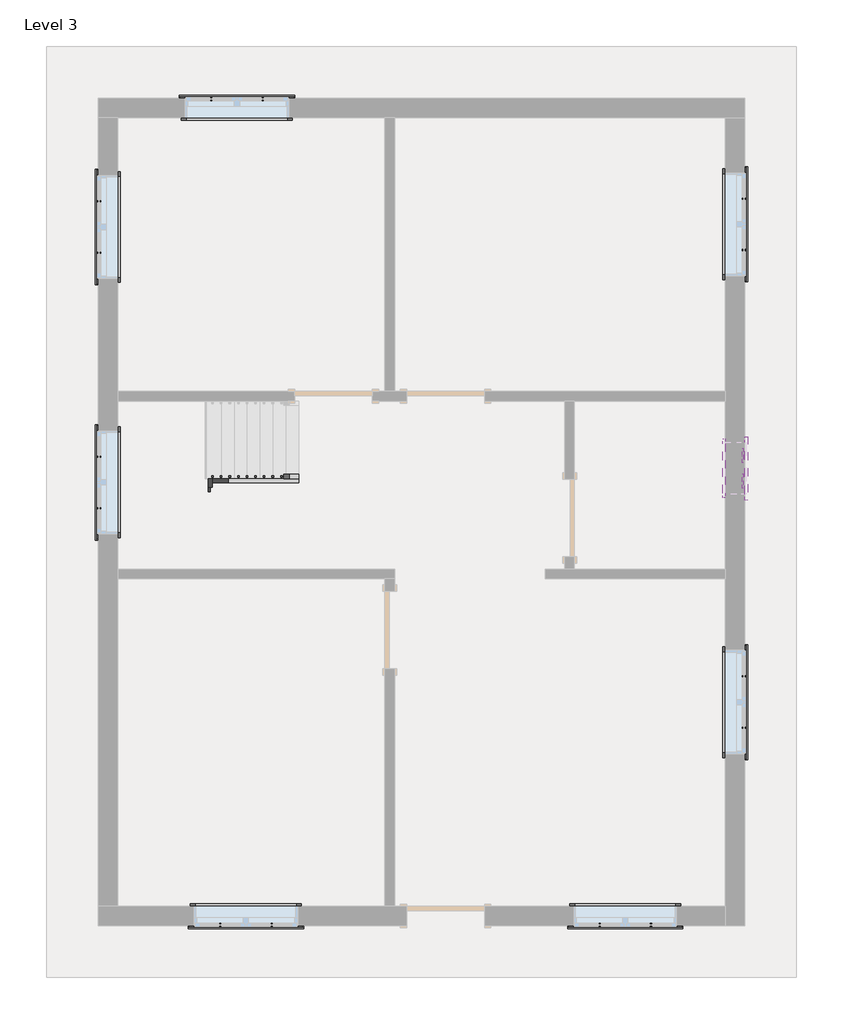
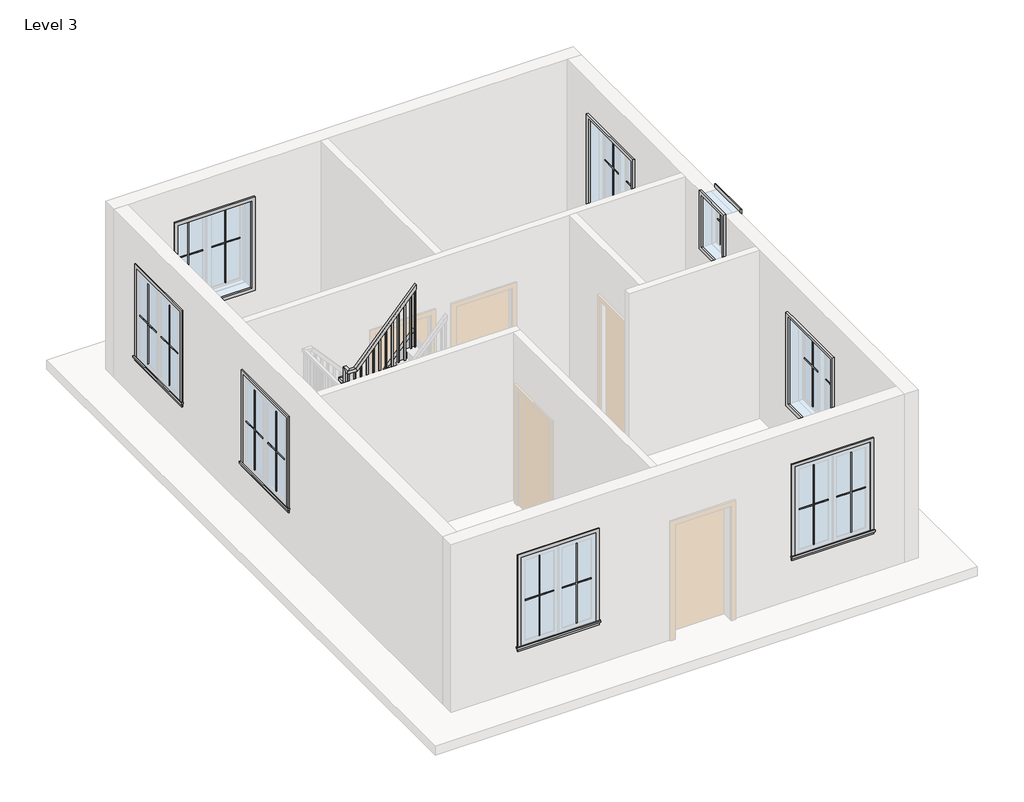
# One storey, part 2 of 2: 32 proxies, 3 members, 1 railing.
"""IFC4 building model written with IfcOpenShell, lengths in millimetres."""

from ifc_helpers import new_model, si_unit, frame, origin, place, context, project, spatial, polyline, outline, extrude, faceted_brep, transform, mapped, element, save
from components import muntin_pattern_2x2_muntin_pattern_2x2_6dad3731, muntin_pattern_2x2_muntin_pattern_2x2_a30a3345, muntin_pattern_2x2_muntin_pattern_2x2_53152e2c, muntin_pattern_2x2_muntin_pattern_2x2_e8f3e573, trim_window_exterior_flat_with_sill_92b9b949, trim_window_exterior_flat_with_sill_a665a915, trim_window_interior_flat_picture_frame_3bb882cf, trim_window_interior_flat_picture_frame_d485c387

model = new_model("IFC4")

# Units and contexts
model_context = context("Model", 3, world=origin())
ifc_project = project(units=[si_unit("LENGTHUNIT", "METRE", prefix="MILLI")], contexts=[model_context])

# Site, building, storey
site = spatial("IfcSite", under=ifc_project)
building = spatial("IfcBuilding", under=site)
storey = spatial("IfcBuildingStorey", under=building, Name="Level 3", Elevation=6096.0)

# Proxies
placement = place(None, origin())
muntin_pattern_2x2_muntin_pattern_2x2_shape = muntin_pattern_2x2_muntin_pattern_2x2_6dad3731(model_context)
element("IfcBuildingElementProxy", 1, Name="Muntin Pattern_2x2 : Muntin Pattern_2x2", ObjectType="Muntin Pattern_2x2 : Muntin Pattern_2x2", at=placement, inside=storey, context=model_context, shape_type="MappedRepresentation", body=[
    mapped(muntin_pattern_2x2_muntin_pattern_2x2_shape, transform((7785.1, 4733.925, 7080.25), x_axis=(-1.0, 0.0, 0.0), y_axis=(0.0, -1.0, 0.0), z_axis=(0.0, 0.0, 1.0))),
])
element("IfcBuildingElementProxy", 2, Name="Muntin Pattern_2x2 : Muntin Pattern_2x2", ObjectType="Muntin Pattern_2x2 : Muntin Pattern_2x2", at=placement, inside=storey, context=model_context, shape_type="MappedRepresentation", body=[
    mapped(muntin_pattern_2x2_muntin_pattern_2x2_shape, transform((3313.1125, 4733.925, 7080.25), x_axis=(-1.0, 0.0, 0.0), y_axis=(0.0, -1.0, 0.0), z_axis=(0.0, 0.0, 1.0))),
])
element("IfcBuildingElementProxy", 3, Name="Muntin Pattern_2x2 : Muntin Pattern_2x2", ObjectType="Muntin Pattern_2x2 : Muntin Pattern_2x2", at=placement, inside=storey, context=model_context, shape_type="MappedRepresentation", body=[
    mapped(muntin_pattern_2x2_muntin_pattern_2x2_shape, transform((8880.475, 13295.3125, 7080.25), x_axis=(0.0, -1.0, 0.0), y_axis=(1.0, 0.0, 0.0), z_axis=(0.0, 0.0, 1.0))),
])
element("IfcBuildingElementProxy", 4, Name="Muntin Pattern_2x2 : Muntin Pattern_2x2", ObjectType="Muntin Pattern_2x2 : Muntin Pattern_2x2", at=placement, inside=storey, context=model_context, shape_type="MappedRepresentation", body=[
    mapped(muntin_pattern_2x2_muntin_pattern_2x2_shape, transform((8880.475, 7662.8625, 7080.25), x_axis=(0.0, -1.0, 0.0), y_axis=(1.0, 0.0, 0.0), z_axis=(0.0, 0.0, 1.0))),
])
element("IfcBuildingElementProxy", 5, Name="Muntin Pattern_2x2 : Muntin Pattern_2x2", ObjectType="Muntin Pattern_2x2 : Muntin Pattern_2x2", at=placement, inside=storey, context=model_context, shape_type="MappedRepresentation", body=[
    mapped(muntin_pattern_2x2_muntin_pattern_2x2_shape, transform((1279.525, 12657.1375, 7080.25), x_axis=(0.0, 1.0, 0.0), y_axis=(-1.0, 0.0, 0.0), z_axis=(0.0, 0.0, 1.0))),
])
element("IfcBuildingElementProxy", 6, Name="Muntin Pattern_2x2 : Muntin Pattern_2x2", ObjectType="Muntin Pattern_2x2 : Muntin Pattern_2x2", at=placement, inside=storey, context=model_context, shape_type="MappedRepresentation", body=[
    mapped(muntin_pattern_2x2_muntin_pattern_2x2_shape, transform((1279.525, 9647.2375, 7080.25), x_axis=(0.0, 1.0, 0.0), y_axis=(-1.0, 0.0, 0.0), z_axis=(0.0, 0.0, 1.0))),
])
element("IfcBuildingElementProxy", 7, Name="Muntin Pattern_2x2 : Muntin Pattern_2x2", ObjectType="Muntin Pattern_2x2 : Muntin Pattern_2x2", at=placement, inside=storey, context=model_context, shape_type="MappedRepresentation", body=[
    mapped(muntin_pattern_2x2_muntin_pattern_2x2_shape, transform((2601.9125, 14468.475, 7080.25), x_axis=(1.0, 0.0, 0.0), y_axis=(0.0, 1.0, 0.0), z_axis=(0.0, 0.0, 1.0))),
])
muntin_pattern_2x2_muntin_pattern_2x2_2_shape = muntin_pattern_2x2_muntin_pattern_2x2_a30a3345(model_context)
element("IfcBuildingElementProxy", 8, Name="Muntin Pattern_2x2 : Muntin Pattern_2x2", ObjectType="Muntin Pattern_2x2 : Muntin Pattern_2x2", at=placement, inside=storey, context=model_context, shape_type="MappedRepresentation", body=[
    mapped(muntin_pattern_2x2_muntin_pattern_2x2_2_shape, transform((7178.675, 4733.925, 7080.25), x_axis=(1.0, 0.0, 0.0), y_axis=(0.0, 1.0, 0.0), z_axis=(0.0, 0.0, 1.0))),
])
element("IfcBuildingElementProxy", 9, Name="Muntin Pattern_2x2 : Muntin Pattern_2x2", ObjectType="Muntin Pattern_2x2 : Muntin Pattern_2x2", at=placement, inside=storey, context=model_context, shape_type="MappedRepresentation", body=[
    mapped(muntin_pattern_2x2_muntin_pattern_2x2_2_shape, transform((2706.6875, 4733.925, 7080.25), x_axis=(1.0, 0.0, 0.0), y_axis=(0.0, 1.0, 0.0), z_axis=(0.0, 0.0, 1.0))),
])
element("IfcBuildingElementProxy", 10, Name="Muntin Pattern_2x2 : Muntin Pattern_2x2", ObjectType="Muntin Pattern_2x2 : Muntin Pattern_2x2", at=placement, inside=storey, context=model_context, shape_type="MappedRepresentation", body=[
    mapped(muntin_pattern_2x2_muntin_pattern_2x2_2_shape, transform((8880.475, 12688.8875, 7080.25), x_axis=(0.0, 1.0, 0.0), y_axis=(-1.0, 0.0, 0.0), z_axis=(0.0, 0.0, 1.0))),
])
element("IfcBuildingElementProxy", 11, Name="Muntin Pattern_2x2 : Muntin Pattern_2x2", ObjectType="Muntin Pattern_2x2 : Muntin Pattern_2x2", at=placement, inside=storey, context=model_context, shape_type="MappedRepresentation", body=[
    mapped(muntin_pattern_2x2_muntin_pattern_2x2_2_shape, transform((8880.475, 7056.4375, 7080.25), x_axis=(0.0, 1.0, 0.0), y_axis=(-1.0, 0.0, 0.0), z_axis=(0.0, 0.0, 1.0))),
])
element("IfcBuildingElementProxy", 12, Name="Muntin Pattern_2x2 : Muntin Pattern_2x2", ObjectType="Muntin Pattern_2x2 : Muntin Pattern_2x2", at=placement, inside=storey, context=model_context, shape_type="MappedRepresentation", body=[
    mapped(muntin_pattern_2x2_muntin_pattern_2x2_2_shape, transform((1279.525, 13263.5625, 7080.25), x_axis=(0.0, -1.0, 0.0), y_axis=(1.0, 0.0, 0.0), z_axis=(0.0, 0.0, 1.0))),
])
element("IfcBuildingElementProxy", 13, Name="Muntin Pattern_2x2 : Muntin Pattern_2x2", ObjectType="Muntin Pattern_2x2 : Muntin Pattern_2x2", at=placement, inside=storey, context=model_context, shape_type="MappedRepresentation", body=[
    mapped(muntin_pattern_2x2_muntin_pattern_2x2_2_shape, transform((1279.525, 10253.6625, 7080.25), x_axis=(0.0, -1.0, 0.0), y_axis=(1.0, 0.0, 0.0), z_axis=(0.0, 0.0, 1.0))),
])
element("IfcBuildingElementProxy", 14, Name="Muntin Pattern_2x2 : Muntin Pattern_2x2", ObjectType="Muntin Pattern_2x2 : Muntin Pattern_2x2", at=placement, inside=storey, context=model_context, shape_type="MappedRepresentation", body=[
    mapped(muntin_pattern_2x2_muntin_pattern_2x2_2_shape, transform((3208.3375, 14468.475, 7080.25), x_axis=(-1.0, 0.0, 0.0), y_axis=(0.0, -1.0, 0.0), z_axis=(0.0, 0.0, 1.0))),
])
muntin_pattern_2x2_muntin_pattern_2x2_3_shape = muntin_pattern_2x2_muntin_pattern_2x2_53152e2c(model_context)
element("IfcBuildingElementProxy", 15, Name="Muntin Pattern_2x2 : Muntin Pattern_2x2", ObjectType="Muntin Pattern_2x2 : Muntin Pattern_2x2", at=placement, inside=storey, context=model_context, shape_type="MappedRepresentation", body=[
    mapped(muntin_pattern_2x2_muntin_pattern_2x2_3_shape, transform((8880.475, 10266.3625, 8299.45), x_axis=(0.0, -1.0, 0.0), y_axis=(1.0, 0.0, 0.0), z_axis=(0.0, 0.0, 1.0))),
])
muntin_pattern_2x2_muntin_pattern_2x2_4_shape = muntin_pattern_2x2_muntin_pattern_2x2_e8f3e573(model_context)
element("IfcBuildingElementProxy", 16, Name="Muntin Pattern_2x2 : Muntin Pattern_2x2", ObjectType="Muntin Pattern_2x2 : Muntin Pattern_2x2", at=placement, inside=storey, context=model_context, shape_type="MappedRepresentation", body=[
    mapped(muntin_pattern_2x2_muntin_pattern_2x2_4_shape, transform((8880.475, 9964.7375, 8299.45), x_axis=(0.0, 1.0, 0.0), y_axis=(-1.0, 0.0, 0.0), z_axis=(0.0, 0.0, 1.0))),
])
trim_window_exterior_flat_with_sill_shape = trim_window_exterior_flat_with_sill_92b9b949(model_context)
element("IfcBuildingElementProxy", 17, Name="Trim-Window-Exterior-Flat : with Sill", ObjectType="Trim-Window-Exterior-Flat : with Sill", at=placement, inside=storey, context=model_context, shape_type="MappedRepresentation", body=[
    mapped(trim_window_exterior_flat_with_sill_shape, transform((7481.8875, 4724.4, 8534.4), x_axis=(1.0, 0.0, 0.0), y_axis=(0.0, 0.0, 1.0), z_axis=(0.0, -1.0, 0.0))),
])
element("IfcBuildingElementProxy", 18, Name="Trim-Window-Exterior-Flat : with Sill", ObjectType="Trim-Window-Exterior-Flat : with Sill", at=placement, inside=storey, context=model_context, shape_type="MappedRepresentation", body=[
    mapped(trim_window_exterior_flat_with_sill_shape, transform((3009.9, 4724.4, 8534.4), x_axis=(1.0, 0.0, 0.0), y_axis=(0.0, 0.0, 1.0), z_axis=(0.0, -1.0, 0.0))),
])
element("IfcBuildingElementProxy", 19, Name="Trim-Window-Exterior-Flat : with Sill", ObjectType="Trim-Window-Exterior-Flat : with Sill", at=placement, inside=storey, context=model_context, shape_type="MappedRepresentation", body=[
    mapped(trim_window_exterior_flat_with_sill_shape, transform((8890.0, 12992.1, 8534.4), x_axis=(0.0, 1.0, 0.0), y_axis=(0.0, 0.0, 1.0), z_axis=(1.0, 0.0, 0.0))),
])
element("IfcBuildingElementProxy", 20, Name="Trim-Window-Exterior-Flat : with Sill", ObjectType="Trim-Window-Exterior-Flat : with Sill", at=placement, inside=storey, context=model_context, shape_type="MappedRepresentation", body=[
    mapped(trim_window_exterior_flat_with_sill_shape, transform((8890.0, 7359.65, 8534.4), x_axis=(0.0, 1.0, 0.0), y_axis=(0.0, 0.0, 1.0), z_axis=(1.0, 0.0, 0.0))),
])
element("IfcBuildingElementProxy", 21, Name="Trim-Window-Exterior-Flat : with Sill", ObjectType="Trim-Window-Exterior-Flat : with Sill", at=placement, inside=storey, context=model_context, shape_type="MappedRepresentation", body=[
    mapped(trim_window_exterior_flat_with_sill_shape, transform((1270.0, 12960.35, 8534.4), x_axis=(0.0, -1.0, 0.0), y_axis=(0.0, 0.0, 1.0), z_axis=(-1.0, 0.0, 0.0))),
])
element("IfcBuildingElementProxy", 22, Name="Trim-Window-Exterior-Flat : with Sill", ObjectType="Trim-Window-Exterior-Flat : with Sill", at=placement, inside=storey, context=model_context, shape_type="MappedRepresentation", body=[
    mapped(trim_window_exterior_flat_with_sill_shape, transform((1270.0, 9950.45, 8534.4), x_axis=(0.0, -1.0, 0.0), y_axis=(0.0, 0.0, 1.0), z_axis=(-1.0, 0.0, 0.0))),
])
element("IfcBuildingElementProxy", 23, Name="Trim-Window-Exterior-Flat : with Sill", ObjectType="Trim-Window-Exterior-Flat : with Sill", at=placement, inside=storey, context=model_context, shape_type="MappedRepresentation", body=[
    mapped(trim_window_exterior_flat_with_sill_shape, transform((2905.125, 14478.0, 8534.4), x_axis=(-1.0, 0.0, 0.0), y_axis=(0.0, 0.0, 1.0), z_axis=(0.0, 1.0, 0.0))),
])
trim_window_exterior_flat_with_sill_2_shape = trim_window_exterior_flat_with_sill_a665a915(model_context)
element("IfcBuildingElementProxy", 24, Name="Trim-Window-Exterior-Flat : with Sill", ObjectType="Trim-Window-Exterior-Flat : with Sill", at=placement, inside=storey, context=model_context, shape_type="MappedRepresentation", body=[
    mapped(trim_window_exterior_flat_with_sill_2_shape, transform((8890.0, 10115.55, 9144.0), x_axis=(0.0, 1.0, 0.0), y_axis=(0.0, 0.0, 1.0), z_axis=(1.0, 0.0, 0.0))),
])
trim_window_interior_flat_picture_frame_shape = trim_window_interior_flat_picture_frame_3bb882cf(model_context)
element("IfcBuildingElementProxy", 25, Name="Trim-Window-Interior-Flat : Picture Frame", ObjectType="Trim-Window-Interior-Flat : Picture Frame", at=placement, inside=storey, context=model_context, shape_type="MappedRepresentation", body=[
    mapped(trim_window_interior_flat_picture_frame_shape, transform((7481.8875, 4953.0, 8534.4), x_axis=(-1.0, 0.0, 0.0), y_axis=(0.0, 0.0, 1.0), z_axis=(0.0, 1.0, 0.0))),
])
element("IfcBuildingElementProxy", 26, Name="Trim-Window-Interior-Flat : Picture Frame", ObjectType="Trim-Window-Interior-Flat : Picture Frame", at=placement, inside=storey, context=model_context, shape_type="MappedRepresentation", body=[
    mapped(trim_window_interior_flat_picture_frame_shape, transform((3009.9, 4953.0, 8534.4), x_axis=(-1.0, 0.0, 0.0), y_axis=(0.0, 0.0, 1.0), z_axis=(0.0, 1.0, 0.0))),
])
element("IfcBuildingElementProxy", 27, Name="Trim-Window-Interior-Flat : Picture Frame", ObjectType="Trim-Window-Interior-Flat : Picture Frame", at=placement, inside=storey, context=model_context, shape_type="MappedRepresentation", body=[
    mapped(trim_window_interior_flat_picture_frame_shape, transform((8661.4, 12992.1, 8534.4), x_axis=(0.0, -1.0, 0.0), y_axis=(0.0, 0.0, 1.0), z_axis=(-1.0, 0.0, 0.0))),
])
element("IfcBuildingElementProxy", 28, Name="Trim-Window-Interior-Flat : Picture Frame", ObjectType="Trim-Window-Interior-Flat : Picture Frame", at=placement, inside=storey, context=model_context, shape_type="MappedRepresentation", body=[
    mapped(trim_window_interior_flat_picture_frame_shape, transform((8661.4, 7359.65, 8534.4), x_axis=(0.0, -1.0, 0.0), y_axis=(0.0, 0.0, 1.0), z_axis=(-1.0, 0.0, 0.0))),
])
element("IfcBuildingElementProxy", 29, Name="Trim-Window-Interior-Flat : Picture Frame", ObjectType="Trim-Window-Interior-Flat : Picture Frame", at=placement, inside=storey, context=model_context, shape_type="MappedRepresentation", body=[
    mapped(trim_window_interior_flat_picture_frame_shape, transform((1498.6, 12960.35, 8534.4), x_axis=(0.0, 1.0, 0.0), y_axis=(0.0, 0.0, 1.0), z_axis=(1.0, 0.0, 0.0))),
])
element("IfcBuildingElementProxy", 30, Name="Trim-Window-Interior-Flat : Picture Frame", ObjectType="Trim-Window-Interior-Flat : Picture Frame", at=placement, inside=storey, context=model_context, shape_type="MappedRepresentation", body=[
    mapped(trim_window_interior_flat_picture_frame_shape, transform((1498.6, 9950.45, 8534.4), x_axis=(0.0, 1.0, 0.0), y_axis=(0.0, 0.0, 1.0), z_axis=(1.0, 0.0, 0.0))),
])
element("IfcBuildingElementProxy", 31, Name="Trim-Window-Interior-Flat : Picture Frame", ObjectType="Trim-Window-Interior-Flat : Picture Frame", at=placement, inside=storey, context=model_context, shape_type="MappedRepresentation", body=[
    mapped(trim_window_interior_flat_picture_frame_shape, transform((2905.125, 14249.4, 8534.4), x_axis=(1.0, 0.0, 0.0), y_axis=(0.0, 0.0, 1.0), z_axis=(0.0, -1.0, 0.0))),
])
trim_window_interior_flat_picture_frame_2_shape = trim_window_interior_flat_picture_frame_d485c387(model_context)
element("IfcBuildingElementProxy", 32, Name="Trim-Window-Interior-Flat : Picture Frame", ObjectType="Trim-Window-Interior-Flat : Picture Frame", at=placement, inside=storey, context=model_context, shape_type="MappedRepresentation", body=[
    mapped(trim_window_interior_flat_picture_frame_2_shape, transform((8661.4, 10115.55, 9144.0), x_axis=(0.0, -1.0, 0.0), y_axis=(0.0, 0.0, 1.0), z_axis=(-1.0, 0.0, 0.0))),
])

# Members
element("IfcMember", 33, ObjectType="Stringer - 2\" Width", at=placement, inside=storey, context=model_context, shape_type="SweptSolid", body=[
    extrude(outline(polyline([(6096.0, 3632.2), (6370.6288314, 3632.2), (7499.5177203, 2616.2), (7043.8883192, 2616.2), (6096.0, 3469.2994873), (6096.0, 3632.2)])), frame((0.0, 9944.1, 0.0), z_axis=(0.0, 1.0, 0.0), x_axis=(0.0, 0.0, 1.0)), (0.0, 0.0, 1.0), 50.8),
])
element("IfcMember", 34, ObjectType="Stringer - 2\" Width", at=placement, inside=storey, context=model_context, shape_type="SweptSolid", body=[
    extrude(outline(polyline([(2565.4, 9994.9), (2616.2, 9994.9), (2616.2, 9893.3), (2565.4, 9893.3), (2565.4, 9994.9)])), frame((0.0, 0.0, 7222.0666667), z_axis=(0.0, 0.0, 1.0), x_axis=(1.0, 0.0, 0.0)), (0.0, 0.0, 1.0), 304.8),
])
element("IfcMember", 35, ObjectType="Stringer - 2\" Width", at=placement, inside=storey, context=model_context, shape_type="SweptSolid", body=[
    extrude(outline(polyline([(7725.2954981, 2565.4), (7269.666097, 2565.4), (8454.9994303, 3632.2), (8910.6288314, 3632.2), (7725.2954981, 2565.4)])), frame((0.0, 9842.5, 0.0), z_axis=(0.0, 1.0, 0.0), x_axis=(0.0, 0.0, 1.0)), (0.0, 0.0, 1.0), 50.8),
])

# Railing
element("IfcRailing", 36, ObjectType="Handrail - Rectangular", at=placement, inside=storey, context=model_context, shape_type="SolidModel", body=[
    faceted_brep([(3632.2, 9994.9, 7179.7333333), (3632.2, 9994.9, 7103.7950998), (3632.2, 10045.7, 7103.7950998), (3632.2, 10045.7, 7179.7333333), (2641.6, 9994.9, 8280.4), (2590.8, 9994.9, 8260.9062109), (2590.8, 10045.7, 8260.9062109), (2641.6, 10045.7, 8280.4), (2641.6, 9994.9, 8365.0666667), (2590.8, 9994.9, 8314.2666667), (2590.8, 10045.7, 8314.2666667), (2641.6, 10045.7, 8365.0666667), (2565.4, 9994.9, 8365.0666667), (2565.4, 9994.9, 8314.2666667), (2514.6, 10045.7, 8314.2666667), (2514.6, 10045.7, 8365.0666667), (2565.4, 9918.7, 8365.0666667), (2565.4, 9867.9, 8314.2666667), (2514.6, 9867.9, 8314.2666667), (2514.6, 9918.7, 8365.0666667), (2565.4, 9918.7, 8619.0666667), (2565.4, 9867.9, 8568.2666667), (2514.6, 9867.9, 8568.2666667), (2514.6, 9918.7, 8619.0666667), (2565.4, 9842.5, 8619.0666667), (2565.4, 9842.5, 8568.2666667), (2514.6, 9791.7, 8568.2666667), (2514.6, 9791.7, 8619.0666667), (2641.6, 9842.5, 8619.0666667), (2664.2244102, 9842.5, 8568.2666667), (2664.2244102, 9791.7, 8568.2666667), (2641.6, 9791.7, 8619.0666667), (3632.2, 9842.5, 9719.7333333), (3632.2, 9791.7, 9719.7333333), (3632.2, 9791.7, 9643.7950998), (3632.2, 9842.5, 9643.7950998)], [[[0, 1, 2, 3]], [[1, 0, 4, 5]], [[2, 1, 5, 6]], [[3, 2, 6, 7]], [[0, 3, 7, 4]], [[5, 4, 8, 9]], [[6, 5, 9, 10]], [[7, 6, 10, 11]], [[4, 7, 11, 8]], [[9, 8, 12, 13]], [[10, 9, 13, 14]], [[11, 10, 14, 15]], [[8, 11, 15, 12]], [[13, 12, 16, 17]], [[14, 13, 17, 18]], [[15, 14, 18, 19]], [[12, 15, 19, 16]], [[17, 16, 20, 21]], [[18, 17, 21, 22]], [[19, 18, 22, 23]], [[16, 19, 23, 20]], [[21, 20, 24, 25]], [[22, 21, 25, 26]], [[23, 22, 26, 27]], [[20, 23, 27, 24]], [[25, 24, 28, 29]], [[26, 25, 29, 30]], [[27, 26, 30, 31]], [[24, 27, 31, 28]], [[32, 33, 34, 35]], [[29, 28, 32, 35]], [[30, 29, 35, 34]], [[31, 30, 34, 33]], [[28, 31, 33, 32]]]),
    extrude(outline(polyline([(9548.5450998, 3546.475), (8636.0, 3546.475), (8636.0, 3565.525), (9569.7117665, 3565.525), (9548.5450998, 3546.475)])), frame((0.0, 9807.575, 0.0), z_axis=(0.0, 1.0, 0.0), x_axis=(0.0, 0.0, 1.0)), (0.0, 0.0, 1.0), 19.05),
    extrude(outline(polyline([(9435.6562109, 3444.875), (8466.6666667, 3444.875), (8466.6666667, 3463.925), (9456.8228776, 3463.925), (9435.6562109, 3444.875)])), frame((0.0, 9807.575, 0.0), z_axis=(0.0, 1.0, 0.0), x_axis=(0.0, 0.0, 1.0)), (0.0, 0.0, 1.0), 19.05),
    extrude(outline(polyline([(9322.767322, 3343.275), (8466.6666667, 3343.275), (8466.6666667, 3362.325), (9343.9339887, 3362.325), (9322.767322, 3343.275)])), frame((0.0, 9807.575, 0.0), z_axis=(0.0, 1.0, 0.0), x_axis=(0.0, 0.0, 1.0)), (0.0, 0.0, 1.0), 19.05),
    extrude(outline(polyline([(9209.8784332, 3241.675), (8297.3333333, 3241.675), (8297.3333333, 3260.725), (9231.0450998, 3260.725), (9209.8784332, 3241.675)])), frame((0.0, 9807.575, 0.0), z_axis=(0.0, 1.0, 0.0), x_axis=(0.0, 0.0, 1.0)), (0.0, 0.0, 1.0), 19.05),
    extrude(outline(polyline([(9096.9895443, 3140.075), (8128.0, 3140.075), (8128.0, 3159.125), (9118.1562109, 3159.125), (9096.9895443, 3140.075)])), frame((0.0, 9807.575, 0.0), z_axis=(0.0, 1.0, 0.0), x_axis=(0.0, 0.0, 1.0)), (0.0, 0.0, 1.0), 19.05),
    extrude(outline(polyline([(8984.1006554, 3038.475), (8128.0, 3038.475), (8128.0, 3057.525), (9005.267322, 3057.525), (8984.1006554, 3038.475)])), frame((0.0, 9807.575, 0.0), z_axis=(0.0, 1.0, 0.0), x_axis=(0.0, 0.0, 1.0)), (0.0, 0.0, 1.0), 19.05),
    extrude(outline(polyline([(8871.2117665, 2936.875), (7958.6666667, 2936.875), (7958.6666667, 2955.925), (8892.3784332, 2955.925), (8871.2117665, 2936.875)])), frame((0.0, 9807.575, 0.0), z_axis=(0.0, 1.0, 0.0), x_axis=(0.0, 0.0, 1.0)), (0.0, 0.0, 1.0), 19.05),
    extrude(outline(polyline([(8758.3228776, 2835.275), (7789.3333333, 2835.275), (7789.3333333, 2854.325), (8779.4895443, 2854.325), (8758.3228776, 2835.275)])), frame((0.0, 9807.575, 0.0), z_axis=(0.0, 1.0, 0.0), x_axis=(0.0, 0.0, 1.0)), (0.0, 0.0, 1.0), 19.05),
    extrude(outline(polyline([(8645.4339887, 2733.675), (7789.3333333, 2733.675), (7789.3333333, 2752.725), (8666.6006554, 2752.725), (8645.4339887, 2733.675)])), frame((0.0, 9807.575, 0.0), z_axis=(0.0, 1.0, 0.0), x_axis=(0.0, 0.0, 1.0)), (0.0, 0.0, 1.0), 19.05),
    extrude(outline(polyline([(8532.5450998, 2632.075), (7620.0, 2632.075), (7620.0, 2651.125), (8553.7117665, 2651.125), (8532.5450998, 2632.075)])), frame((0.0, 9807.575, 0.0), z_axis=(0.0, 1.0, 0.0), x_axis=(0.0, 0.0, 1.0)), (0.0, 0.0, 1.0), 19.05),
    extrude(outline(polyline([(2549.525, 9928.225), (2549.525, 9909.175), (2530.475, 9909.175), (2530.475, 9928.225), (2549.525, 9928.225)])), frame((0.0, 0.0, 7450.6666667), z_axis=(0.0, 0.0, 1.0), x_axis=(1.0, 0.0, 0.0)), (0.0, 0.0, 1.0), 863.6),
    extrude(outline(polyline([(2625.725, 10010.775), (2606.675, 10010.775), (2606.675, 10029.825), (2625.725, 10029.825), (2625.725, 10010.775)])), frame((0.0, 0.0, 7281.3333333), z_axis=(0.0, 0.0, 1.0), x_axis=(1.0, 0.0, 0.0)), (0.0, 0.0, 1.0), 1032.9333333),
    extrude(outline(polyline([(8130.3784332, 2708.275), (7281.3333333, 2708.275), (7281.3333333, 2727.325), (8109.2117665, 2727.325), (8130.3784332, 2708.275)])), frame((0.0, 10010.775, 0.0), z_axis=(0.0, 1.0, 0.0), x_axis=(0.0, 0.0, 1.0)), (0.0, 0.0, 1.0), 19.05),
    extrude(outline(polyline([(8017.4895443, 2809.875), (7112.0, 2809.875), (7112.0, 2828.925), (7996.3228776, 2828.925), (8017.4895443, 2809.875)])), frame((0.0, 10010.775, 0.0), z_axis=(0.0, 1.0, 0.0), x_axis=(0.0, 0.0, 1.0)), (0.0, 0.0, 1.0), 19.05),
    extrude(outline(polyline([(7904.6006554, 2911.475), (6942.6666667, 2911.475), (6942.6666667, 2930.525), (7883.4339887, 2930.525), (7904.6006554, 2911.475)])), frame((0.0, 10010.775, 0.0), z_axis=(0.0, 1.0, 0.0), x_axis=(0.0, 0.0, 1.0)), (0.0, 0.0, 1.0), 19.05),
    extrude(outline(polyline([(7791.7117665, 3013.075), (6942.6666667, 3013.075), (6942.6666667, 3032.125), (7770.5450998, 3032.125), (7791.7117665, 3013.075)])), frame((0.0, 10010.775, 0.0), z_axis=(0.0, 1.0, 0.0), x_axis=(0.0, 0.0, 1.0)), (0.0, 0.0, 1.0), 19.05),
    extrude(outline(polyline([(7678.8228776, 3114.675), (6773.3333333, 3114.675), (6773.3333333, 3133.725), (7657.6562109, 3133.725), (7678.8228776, 3114.675)])), frame((0.0, 10010.775, 0.0), z_axis=(0.0, 1.0, 0.0), x_axis=(0.0, 0.0, 1.0)), (0.0, 0.0, 1.0), 19.05),
    extrude(outline(polyline([(7565.9339887, 3216.275), (6604.0, 3216.275), (6604.0, 3235.325), (7544.767322, 3235.325), (7565.9339887, 3216.275)])), frame((0.0, 10010.775, 0.0), z_axis=(0.0, 1.0, 0.0), x_axis=(0.0, 0.0, 1.0)), (0.0, 0.0, 1.0), 19.05),
    extrude(outline(polyline([(7453.0450998, 3317.875), (6604.0, 3317.875), (6604.0, 3336.925), (7431.8784332, 3336.925), (7453.0450998, 3317.875)])), frame((0.0, 10010.775, 0.0), z_axis=(0.0, 1.0, 0.0), x_axis=(0.0, 0.0, 1.0)), (0.0, 0.0, 1.0), 19.05),
    extrude(outline(polyline([(7340.1562109, 3419.475), (6434.6666667, 3419.475), (6434.6666667, 3438.525), (7318.9895443, 3438.525), (7340.1562109, 3419.475)])), frame((0.0, 10010.775, 0.0), z_axis=(0.0, 1.0, 0.0), x_axis=(0.0, 0.0, 1.0)), (0.0, 0.0, 1.0), 19.05),
    extrude(outline(polyline([(7227.267322, 3521.075), (6265.3333333, 3521.075), (6265.3333333, 3540.125), (7206.1006554, 3540.125), (7227.267322, 3521.075)])), frame((0.0, 10010.775, 0.0), z_axis=(0.0, 1.0, 0.0), x_axis=(0.0, 0.0, 1.0)), (0.0, 0.0, 1.0), 19.05),
    extrude(outline(polyline([(2549.525, 9826.625), (2549.525, 9807.575), (2530.475, 9807.575), (2530.475, 9826.625), (2549.525, 9826.625)])), frame((0.0, 0.0, 7450.6666667), z_axis=(0.0, 0.0, 1.0), x_axis=(1.0, 0.0, 0.0)), (0.0, 0.0, 1.0), 1117.6),
    extrude(outline(polyline([(2549.525, 10010.775), (2530.475, 10010.775), (2530.475, 10029.825), (2549.525, 10029.825), (2549.525, 10010.775)])), frame((0.0, 0.0, 7450.6666667), z_axis=(0.0, 0.0, 1.0), x_axis=(1.0, 0.0, 0.0)), (0.0, 0.0, 1.0), 863.6),
    extrude(outline(polyline([(9622.6284332, 3613.15), (8636.0, 3613.15), (8636.0, 3632.2), (9643.7950998, 3632.2), (9622.6284332, 3613.15)])), frame((0.0, 9807.575, 0.0), z_axis=(0.0, 1.0, 0.0), x_axis=(0.0, 0.0, 1.0)), (0.0, 0.0, 1.0), 19.05),
    extrude(outline(polyline([(7124.9617665, 3613.15), (6265.3333333, 3613.15), (6265.3333333, 3632.2), (7103.7950998, 3632.2), (7124.9617665, 3613.15)])), frame((0.0, 10010.775, 0.0), z_axis=(0.0, 1.0, 0.0), x_axis=(0.0, 0.0, 1.0)), (0.0, 0.0, 1.0), 19.05),
])

save(model, "model.ifc")

# Revit data of these elements
# Type "Muntin Pattern_2x2 : Muntin Pattern_2x2"
#   Width [instance default] = 4' - 0"
#   Thickness = 0' - 0 1/2"
#   Height [instance default] = 4' - 0"
#   Distance = 0' - 0 3/4"
#   Interior Material [instance default] = none
#   Exterior Material [instance default] = none
#   Default Elevation = 0
# Type "Trim-Window-Exterior-Flat : with Sill"
#   Trim Width = 0' - 2 1/4"
#   Trim Thickness_Picture Frame = 0' - 1 1/4"
#   Trim Thickness_with Sill = 0' - 0 3/4"
#   Sill Thickness = 0' - 1 1/4"
#   Opening Width [instance default] = 2' - 0"
#   Opening Height [instance default] = 3' - 0"
#   Default Elevation = 4' - 0"
#   Sill = yes
#   Picture Frame = no
#   Trim Material [instance default] = none
# Type "Trim-Window-Interior-Flat : Picture Frame"
#   Trim Thickness_Picture Frame = 0' - 1 1/4"
#   Trim Width = 0' - 2 1/4"
#   Trim Thickness_with Sill = 0' - 0 3/4"
#   Sill Thickness = 0' - 1 1/4"
#   Opening Width [instance default] = 2' - 0"
#   Opening Height [instance default] = 3' - 0"
#   Default Elevation = 4' - 0"
#   Sill = no
#   Picture Frame = yes
#   Trim Material [instance default] = none
# Type "Handrail - Rectangular"
#   Assembly Code = "C2010400"
#   built-in parameter 1008612 = 0.0416667 (stored number, unit not read)
#   built-in parameter 1008611 = 0.0416667 (stored number, unit not read)
#   built-in parameter 1008609 = 0.333333 (stored number, unit not read)
#   built-in parameter 1008604 = 0.166667 (stored number, unit not read)
#   built-in parameter 1008603 = 0.166667 (stored number, unit not read)
#   Railing Height = 3' - 0"
#   built-in parameter 1008630 = 2
#   built-in parameter 1008610 = 2
#   built-in parameter 1008618 = Baluster - Square : 3/4"
# Elements 1, 2, 3, 4, 5, 6, 7, 8, 9, 10, 11, 12, 13, 14 (IfcBuildingElementProxy, "Muntin Pattern_2x2 : Muntin Pattern_2x2")
#   Width = 1' - 6 5/8"
#   Height = 4' - 6 1/2"
#   Interior Material = Wood - Stained
#   Exterior Material = Clad - White
#   Phase Created = New Construction
#   Materials on its faces: "Clad - White", "Wood - Stained"
# Elements 15, 16 (IfcBuildingElementProxy, "Muntin Pattern_2x2 : Muntin Pattern_2x2")
#   Width = 0' - 6 5/8"
#   Height = 2' - 6 1/2"
#   Interior Material = Wood - Stained
#   Exterior Material = Clad - White
#   Phase Created = New Construction
#   Materials on its faces: "Clad - White", "Wood - Stained"
# Elements 17, 18, 19, 20, 21, 22, 23 (IfcBuildingElementProxy, "Trim-Window-Exterior-Flat : with Sill")
#   Opening Width = 4' - 0"
#   Opening Height = 5' - 0"
#   Trim Material = Clad - White
#   Phase Created = New Construction
#   Materials on its faces: "Clad - White"
# Element 24 (IfcBuildingElementProxy, "Trim-Window-Exterior-Flat : with Sill")
#   Opening Width = 2' - 0"
#   Opening Height = 3' - 0"
#   Trim Material = Clad - White
#   Phase Created = New Construction
#   Materials on its faces: "Clad - White"
# Elements 25, 26, 27, 28, 29, 30, 31 (IfcBuildingElementProxy, "Trim-Window-Interior-Flat : Picture Frame")
#   Opening Width = 4' - 0"
#   Opening Height = 5' - 0"
#   Trim Material = Wood - Stained
#   Phase Created = New Construction
#   Materials on its faces: "Wood - Stained"
# Element 32 (IfcBuildingElementProxy, "Trim-Window-Interior-Flat : Picture Frame")
#   Opening Width = 2' - 0"
#   Opening Height = 3' - 0"
#   Trim Material = Wood - Stained
#   Phase Created = New Construction
#   Materials on its faces: "Wood - Stained"
# Elements 33, 34, 35 (IfcMember, "Stringer - 2\" Width")
#   Phase Created = New Construction
# Element 36 (IfcRailing, "Handrail - Rectangular")
#   Phase Created = New Construction
# Materials
#   "Clad - White": class "Wood", colour RGB 242 242 238, transparency 0, Cost = 0
#   "Wood - Stained": class "Wood", colour RGB 224 178 126, transparency 0, Cost = 0
